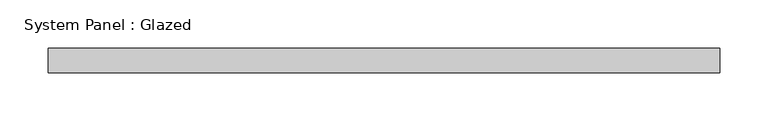
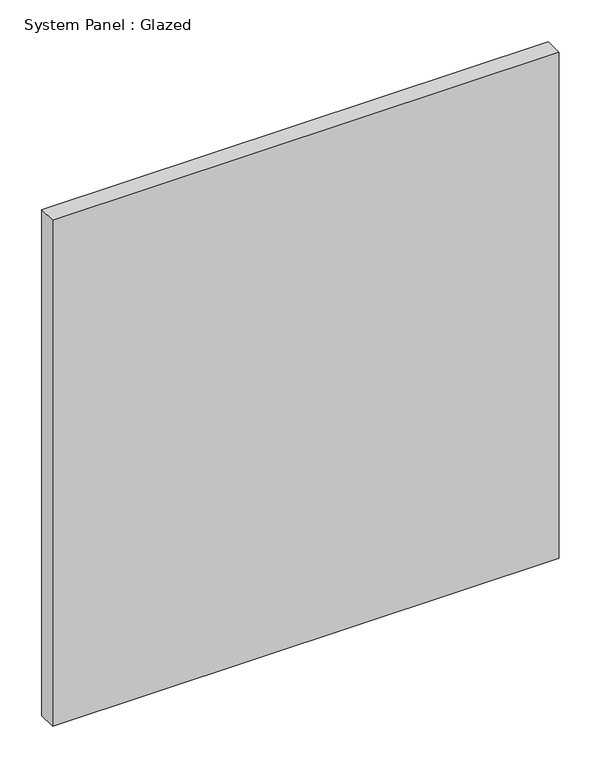
"""IFC4 building model written with IfcOpenShell, lengths in millimetres: plate geometry, System Panel : Glazed."""

from ifc_helpers import new_model, si_unit, origin, origin_with_axes, place, context, project, spatial, polyline, outline, extrude, source, transform, mapped, element, save


def system_panel_glazed_093ce7df(model_context):
    return source(origin(), model_context, "Body", "SweptSolid", [
        extrude(outline(polyline([(349.25, 19.05), (-349.25, 19.05), (-349.25, 44.45), (349.25, 44.45), (349.25, 19.05)])), origin_with_axes(), (0.0, 0.0, 1.0), 737.1888769),
    ])


if __name__ == "__main__":
    model = new_model("IFC4")
    model_context = context("Model", 3, world=origin())
    ifc_project = project(units=[si_unit("LENGTHUNIT", "METRE", prefix="MILLI")], contexts=[model_context])
    site = spatial("IfcSite", under=ifc_project)
    building = spatial("IfcBuilding", under=site)
    placement = place(None, origin())
    system_panel_glazed_shape = system_panel_glazed_093ce7df(model_context)
    element("IfcPlate", 1, ObjectType="System Panel : Glazed", at=placement, inside=building, context=model_context, shape_type="MappedRepresentation", body=[
        mapped(system_panel_glazed_shape, transform((0.0, 0.0, 0.0), x_axis=(1.0, 0.0, 0.0), y_axis=(0.0, 1.0, 0.0), z_axis=(0.0, 0.0, 1.0))),
    ])
    save(model, "model.ifc")

# Revit data of these elements
# Type "System Panel : Glazed"
#   Construction Type Id = "GSP4R"
#   Analytic Construction = "1/8 in Pilkington single glazing"
#   Visual Light Transmittance = 0.9
#   Solar Heat Gain Coefficient = 0.86
#   Heat Transfer Coefficient (U) = 1.18115 BTU/(h·ft²·°F)
#   Define Thermal Properties by = 1
# Element 1 (IfcPlate, "System Panel : Glazed")
#   Materials on its faces: "Glass"
# Materials
#   "Glass": class "Glass", colour RGB 0 128 192, transparency 0.75, Description = "Soda Lime Glass", Cost = 0
